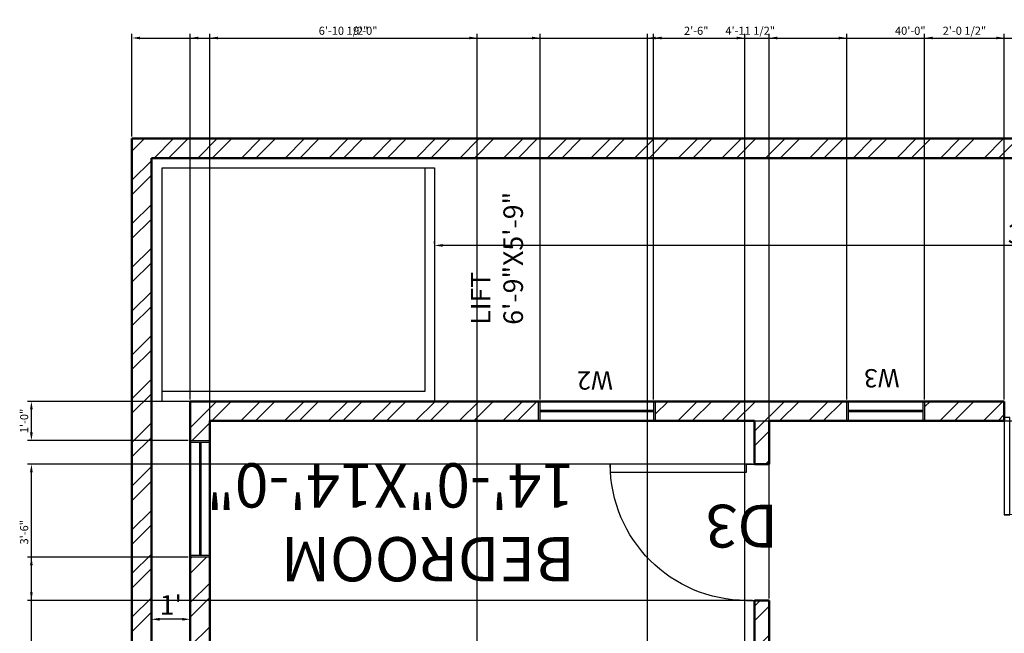
# Model space of a CAD drawing. Units: inches. Extents: x 244 to 2800, y 1060 to 1700.
# Tile 9 of 13: x 1478 to 1781, y 1480 to 1670. Entities that reach past the tile are written whole.
import ezdxf

# ---------------------------------------------------------------- set-up
doc = ezdxf.new("R2010")
doc.units = ezdxf.units.IN
for name, color, linetype, lineweight in [('A-ANNO-DIMS', 2, 'Continuous', 18), ('A-ANNO-TEXT', 1, 'Continuous', 18), ('A-DOOR', 5, 'Continuous', 25), ('A-EQPM', 4, 'Continuous', 25), ('A-GLAZ', 3, 'Continuous', 25), ('A-WALL', 7, 'Continuous', 50), ('A-WALL-PATT', 8, 'Continuous', 13)]:
    doc.layers.add(name, color=color, linetype=linetype, lineweight=lineweight)
doc.styles.get("Standard").update_dxf_attribs({"font": 'arial.ttf'})
doc.dimstyles.new('ISO-25', dxfattribs={"dimtxt": 2.5, "dimasz": 2.5, "dimexe": 1.25, "dimexo": 0.625, "dimtad": 1, "dimlunit": 4, "dimtxsty": 'Standard', "dimcen": 2.5, "dimadec": 0, "dimazin": 0, "dimtfac": 1, "dimtmove": 0, "dimatfit": 3, "dimfxl": 1, "dimarcsym": 0})

# ---------------------------------------------------------------- blocks, each defined once
blk = doc.blocks.new('*U2')
for p, q in [((0, 0), (0, -5)), ((30, 0), (30, -5))]:
    blk.add_line(p, q)
blk.add_lwpolyline([(0, 0), (0, 30), (1.75, 30), (1.75, 0)], close=True)
blk.add_arc((0, 0), 30, 0, 90)
blk = doc.blocks.new('*D29')
at = {"layer": 'A-ANNO-DIMS', "color": 0, "lineweight": -2, "transparency": 16777216}
for p, q in [((1605.7, 1600.68), (1605.7, 1601.31)), ((1983.9, 1600.06), (1608.2, 1600.06)), ((1986.4, 1600.68), (1986.4, 1601.31))]:
    blk.add_line(p, q, dxfattribs=at)
at = {"layer": 'A-ANNO-DIMS', "color": 0, "transparency": 16777216}
for points in [[(1608.2, 1600.47), (1608.2, 1599.64), (1605.7, 1600.06)], [(1983.9, 1600.47), (1983.9, 1599.64), (1986.4, 1600.06)]]:
    blk.add_solid(points, dxfattribs=at)
at = {"layer": 'Defpoints', "color": 0, "transparency": 16777216}
for p in [(1605.7, 1600.06), (1605.7, 1600.06), (1986.4, 1600.06)]:
    blk.add_point(p, dxfattribs=at)
at = {"layer": 'A-ANNO-DIMS', "color": 0, "transparency": 16777216, "insert": (1796.05, 1607.8), "char_height": 6, "attachment_point": 5}
blk.add_mtext('31\'-8{\\H1x;\\S3/4;}"', dxfattribs=at)
blk = doc.blocks.new('*D30')
at = {"layer": 'A-ANNO-DIMS', "color": 0, "lineweight": -2, "transparency": 16777216}
for p, q in [((1518.4, 1482.07), (1518.4, 1486.07)), ((1527.9, 1484.82), (1520.9, 1484.82)), ((1530.4, 1482.07), (1530.4, 1486.07))]:
    blk.add_line(p, q, dxfattribs=at)
at = {"layer": 'A-ANNO-DIMS', "color": 0, "transparency": 16777216}
for points in [[(1520.9, 1485.24), (1520.9, 1484.4), (1518.4, 1484.82)], [(1527.9, 1485.24), (1527.9, 1484.4), (1530.4, 1484.82)]]:
    blk.add_solid(points, dxfattribs=at)
at = {"layer": 'Defpoints', "color": 0, "transparency": 16777216}
for p in [(1518.4, 1484.82), (1518.4, 1481.44), (1530.4, 1481.44)]:
    blk.add_point(p, dxfattribs=at)
at = {"layer": 'A-ANNO-DIMS', "color": 0, "transparency": 16777216, "insert": (1524.4, 1488.46), "char_height": 6, "attachment_point": 5}
blk.add_mtext("1'", dxfattribs=at)
blk = doc.blocks.new('WIN-36')
for p, q in [((0, 0), (0, 6)), ((0, 6), (35.94, 6)), ((35.94, 6), (35.94, 0)), ((35.94, 0), (0, 0))]:
    blk.add_line(p, q)
blk = doc.blocks.new('WIN-24')
for p, q in [((0, 0), (0, 23.94)), ((0, 23.94), (6, 23.94)), ((6, 23.94), (6, 0)), ((6, 0), (0, 0))]:
    blk.add_line(p, q)
blk = doc.blocks.new('LIFT-CAR')
for p, q in [((0, 0), (0, 72)), ((0, 72), (84, 72)), ((81, 72), (81, 3)), ((84, 72), (84, 0)), ((81, 3), (0, 3)), ((84, 0), (0, 0))]:
    blk.add_line(p, q)
blk = doc.blocks.new('*D74')
at = {"layer": 'A-ANNO-DIMS', "color": 0, "lineweight": -2, "transparency": 16777216}
for p, q in [((1512.4, 1633.61), (1512.4, 1665.24)), ((1514.9, 1663.99), (1989.9, 1663.99)), ((1992.4, 1633.61), (1992.4, 1665.24))]:
    blk.add_line(p, q, dxfattribs=at)
at = {"layer": 'A-ANNO-DIMS', "color": 0, "transparency": 16777216}
for points in [[(1514.9, 1664.4), (1514.9, 1663.57), (1512.4, 1663.99)], [(1989.9, 1664.4), (1989.9, 1663.57), (1992.4, 1663.99)]]:
    blk.add_solid(points, dxfattribs=at)
at = {"layer": 'Defpoints', "color": 0, "transparency": 16777216}
for p in [(1992.4, 1663.99), (1512.4, 1632.99), (1992.4, 1632.99)]:
    blk.add_point(p, dxfattribs=at)
at = {"layer": 'A-ANNO-DIMS', "color": 0, "transparency": 16777216, "insert": (1752.4, 1665.89), "char_height": 2.5, "attachment_point": 5}
blk.add_mtext('40\'-0"', dxfattribs=at)
blk = doc.blocks.new('*D76')
at = {"layer": 'A-ANNO-DIMS', "color": 0, "lineweight": -2, "transparency": 16777216}
for p, q in [((1530.4, 1552.61), (1530.4, 1665.24)), ((1532.9, 1663.99), (1635.8, 1663.99)), ((1638.3, 1552.61), (1638.3, 1665.24))]:
    blk.add_line(p, q, dxfattribs=at)
at = {"layer": 'A-ANNO-DIMS', "color": 0, "transparency": 16777216}
for points in [[(1532.9, 1664.4), (1532.9, 1663.57), (1530.4, 1663.99)], [(1635.8, 1664.4), (1635.8, 1663.57), (1638.3, 1663.99)]]:
    blk.add_solid(points, dxfattribs=at)
at = {"layer": 'Defpoints', "color": 0, "transparency": 16777216}
for p in [(1638.3, 1663.99), (1530.4, 1551.99), (1638.3, 1551.99)]:
    blk.add_point(p, dxfattribs=at)
at = {"layer": 'A-ANNO-DIMS', "color": 0, "transparency": 16777216, "insert": (1584.35, 1665.89), "char_height": 2.5, "attachment_point": 5}
blk.add_mtext('9\'-0"', dxfattribs=at)
blk = doc.blocks.new('*D77')
at = {"layer": 'A-ANNO-DIMS', "color": 0, "lineweight": -2, "transparency": 16777216}
for p, q in [((1673.24, 1552.61), (1673.24, 1665.24)), ((1675.74, 1663.99), (1730.36, 1663.99)), ((1732.86, 1552.61), (1732.86, 1665.24))]:
    blk.add_line(p, q, dxfattribs=at)
at = {"layer": 'A-ANNO-DIMS', "color": 0, "transparency": 16777216}
for points in [[(1675.74, 1664.4), (1675.74, 1663.57), (1673.24, 1663.99)], [(1730.36, 1664.4), (1730.36, 1663.57), (1732.86, 1663.99)]]:
    blk.add_solid(points, dxfattribs=at)
at = {"layer": 'Defpoints', "color": 0, "transparency": 16777216}
for p in [(1732.86, 1663.99), (1673.24, 1551.99), (1732.86, 1551.99)]:
    blk.add_point(p, dxfattribs=at)
at = {"layer": 'A-ANNO-DIMS', "color": 0, "transparency": 16777216, "insert": (1703.05, 1665.9), "char_height": 2.5, "attachment_point": 5}
blk.add_mtext('4\'-11 1/2"', dxfattribs=at)
blk = doc.blocks.new('*D78')
at = {"layer": 'A-ANNO-DIMS', "color": 0, "lineweight": -2, "transparency": 16777216}
for p, q in [((1756.81, 1552.61), (1756.81, 1665.24)), ((1759.31, 1663.99), (1778.9, 1663.99)), ((1781.4, 1552.61), (1781.4, 1665.24))]:
    blk.add_line(p, q, dxfattribs=at)
at = {"layer": 'A-ANNO-DIMS', "color": 0, "transparency": 16777216}
for points in [[(1759.31, 1664.4), (1759.31, 1663.57), (1756.81, 1663.99)], [(1778.9, 1664.4), (1778.9, 1663.57), (1781.4, 1663.99)]]:
    blk.add_solid(points, dxfattribs=at)
at = {"layer": 'Defpoints', "color": 0, "transparency": 16777216}
for p in [(1781.4, 1663.99), (1756.81, 1551.99), (1781.4, 1551.99)]:
    blk.add_point(p, dxfattribs=at)
at = {"layer": 'A-ANNO-DIMS', "color": 0, "transparency": 16777216, "insert": (1769.1, 1665.9), "char_height": 2.5, "attachment_point": 5}
blk.add_mtext('2\'-0 1/2"', dxfattribs=at)
blk = doc.blocks.new('*D83')
at = {"layer": 'A-ANNO-DIMS', "color": 0, "lineweight": -2, "transparency": 16777216}
for p, q in [((1529.77, 1503.97), (1480.15, 1503.97)), ((1481.4, 1349.38), (1481.4, 1501.47)), ((1529.77, 1346.88), (1480.15, 1346.88))]:
    blk.add_line(p, q, dxfattribs=at)
at = {"layer": 'A-ANNO-DIMS', "color": 0, "transparency": 16777216}
for points in [[(1480.98, 1501.47), (1481.81, 1501.47), (1481.4, 1503.97)], [(1480.98, 1349.38), (1481.81, 1349.38), (1481.4, 1346.88)]]:
    blk.add_solid(points, dxfattribs=at)
at = {"layer": 'Defpoints', "color": 0, "transparency": 16777216}
for p in [(1481.4, 1503.97), (1530.4, 1503.97), (1530.4, 1346.88)]:
    blk.add_point(p, dxfattribs=at)
at = {"layer": 'A-ANNO-DIMS', "color": 0, "transparency": 16777216, "insert": (1479.49, 1425.42), "char_height": 2.5, "attachment_point": 5, "rotation": 90}
blk.add_mtext('13\'-1"', dxfattribs=at)
blk = doc.blocks.new('*D84')
at = {"layer": 'A-ANNO-DIMS', "color": 0, "lineweight": -2, "transparency": 16777216}
for p, q in [((1529.77, 1551.99), (1480.15, 1551.99)), ((1481.4, 1542.41), (1481.4, 1549.49)), ((1529.77, 1539.91), (1480.15, 1539.91))]:
    blk.add_line(p, q, dxfattribs=at)
at = {"layer": 'A-ANNO-DIMS', "color": 0, "transparency": 16777216}
for points in [[(1480.98, 1549.49), (1481.81, 1549.49), (1481.4, 1551.99)], [(1480.98, 1542.41), (1481.81, 1542.41), (1481.4, 1539.91)]]:
    blk.add_solid(points, dxfattribs=at)
at = {"layer": 'Defpoints', "color": 0, "transparency": 16777216}
for p in [(1481.4, 1551.99), (1530.4, 1551.99), (1530.4, 1539.91)]:
    blk.add_point(p, dxfattribs=at)
at = {"layer": 'A-ANNO-DIMS', "color": 0, "transparency": 16777216, "insert": (1479.49, 1545.95), "char_height": 2.5, "attachment_point": 5, "rotation": 90}
blk.add_mtext('1\'-0"', dxfattribs=at)
blk = doc.blocks.new('*D87')
at = {"layer": 'A-ANNO-DIMS', "color": 0, "lineweight": -2, "transparency": 16777216}
for p, q in [((1537.02, 1545.99), (2024.65, 1545.99)), ((2023.4, 1375.49), (2023.4, 1543.49)), ((1537.02, 1372.99), (2024.65, 1372.99))]:
    blk.add_line(p, q, dxfattribs=at)
at = {"layer": 'A-ANNO-DIMS', "color": 0, "transparency": 16777216}
for points in [[(2022.98, 1543.49), (2023.81, 1543.49), (2023.4, 1545.99)], [(2022.98, 1375.49), (2023.81, 1375.49), (2023.4, 1372.99)]]:
    blk.add_solid(points, dxfattribs=at)
at = {"layer": 'Defpoints', "color": 0, "transparency": 16777216}
for p in [(1536.4, 1545.99), (2023.4, 1545.99), (1536.4, 1372.99)]:
    blk.add_point(p, dxfattribs=at)
at = {"layer": 'A-ANNO-DIMS', "color": 0, "transparency": 16777216, "insert": (2021.49, 1459.49), "char_height": 2.5, "attachment_point": 5, "rotation": 90}
blk.add_mtext('14\'-5"', dxfattribs=at)
blk = doc.blocks.new('*D88')
at = {"layer": 'A-ANNO-DIMS', "color": 0, "lineweight": -2, "transparency": 16777216}
for p, q in [((1536.4, 1373.61), (1536.4, 1665.24)), ((1538.9, 1663.99), (1616.4, 1663.99)), ((1618.9, 1369.11), (1618.9, 1665.24))]:
    blk.add_line(p, q, dxfattribs=at)
at = {"layer": 'A-ANNO-DIMS', "color": 0, "transparency": 16777216}
for points in [[(1538.9, 1664.4), (1538.9, 1663.57), (1536.4, 1663.99)], [(1616.4, 1664.4), (1616.4, 1663.57), (1618.9, 1663.99)]]:
    blk.add_solid(points, dxfattribs=at)
at = {"layer": 'Defpoints', "color": 0, "transparency": 16777216}
for p in [(1618.9, 1663.99), (1536.4, 1372.99), (1618.9, 1368.49)]:
    blk.add_point(p, dxfattribs=at)
at = {"layer": 'A-ANNO-DIMS', "color": 0, "transparency": 16777216, "insert": (1577.65, 1665.9), "char_height": 2.5, "attachment_point": 5}
blk.add_mtext('6\'-10 1/2"', dxfattribs=at)
blk = doc.blocks.new('*D89')
at = {"layer": 'A-ANNO-DIMS', "color": 0, "lineweight": -2, "transparency": 16777216}
for p, q in [((1671.4, 1373.61), (1671.4, 1665.24)), ((1673.9, 1663.99), (1698.9, 1663.99)), ((1701.4, 1373.61), (1701.4, 1665.24))]:
    blk.add_line(p, q, dxfattribs=at)
at = {"layer": 'A-ANNO-DIMS', "color": 0, "transparency": 16777216}
for points in [[(1673.9, 1664.4), (1673.9, 1663.57), (1671.4, 1663.99)], [(1698.9, 1664.4), (1698.9, 1663.57), (1701.4, 1663.99)]]:
    blk.add_solid(points, dxfattribs=at)
at = {"layer": 'Defpoints', "color": 0, "transparency": 16777216}
for p in [(1701.4, 1663.99), (1671.4, 1372.99), (1701.4, 1372.99)]:
    blk.add_point(p, dxfattribs=at)
at = {"layer": 'A-ANNO-DIMS', "color": 0, "transparency": 16777216, "insert": (1686.4, 1665.89), "char_height": 2.5, "attachment_point": 5}
blk.add_mtext('2\'-6"', dxfattribs=at)
blk = doc.blocks.new('*D90')
at = {"layer": 'A-ANNO-DIMS', "color": 0, "lineweight": -2, "transparency": 16777216}
for p, q in [((1708.9, 1491.26), (1708.9, 1665.24)), ((1711.4, 1663.99), (1893.9, 1663.99)), ((1896.4, 1473.26), (1896.4, 1665.24))]:
    blk.add_line(p, q, dxfattribs=at)
at = {"layer": 'A-ANNO-DIMS', "color": 0, "transparency": 16777216}
for points in [[(1711.4, 1664.4), (1711.4, 1663.57), (1708.9, 1663.99)], [(1893.9, 1664.4), (1893.9, 1663.57), (1896.4, 1663.99)]]:
    blk.add_solid(points, dxfattribs=at)
at = {"layer": 'Defpoints', "color": 0, "transparency": 16777216}
for p in [(1896.4, 1663.99), (1708.9, 1490.64), (1896.4, 1472.64)]:
    blk.add_point(p, dxfattribs=at)
at = {"layer": 'A-ANNO-DIMS', "color": 0, "transparency": 16777216, "insert": (1802.65, 1665.9), "char_height": 2.5, "attachment_point": 5}
blk.add_mtext('15\'-7 1/2"', dxfattribs=at)
blk = doc.blocks.new('*D93')
at = {"layer": 'A-ANNO-DIMS', "color": 0, "lineweight": -2, "transparency": 16777216}
for p, q in [((1703.77, 1532.64), (1480.15, 1532.64)), ((1481.4, 1493.14), (1481.4, 1530.14)), ((1703.77, 1490.64), (1480.15, 1490.64))]:
    blk.add_line(p, q, dxfattribs=at)
at = {"layer": 'A-ANNO-DIMS', "color": 0, "transparency": 16777216}
for points in [[(1480.98, 1530.14), (1481.81, 1530.14), (1481.4, 1532.64)], [(1480.98, 1493.14), (1481.81, 1493.14), (1481.4, 1490.64)]]:
    blk.add_solid(points, dxfattribs=at)
at = {"layer": 'Defpoints', "color": 0, "transparency": 16777216}
for p in [(1481.4, 1532.64), (1704.4, 1532.64), (1704.4, 1490.64)]:
    blk.add_point(p, dxfattribs=at)
at = {"layer": 'A-ANNO-DIMS', "color": 0, "transparency": 16777216, "insert": (1479.49, 1511.64), "char_height": 2.5, "attachment_point": 5, "rotation": 90}
blk.add_mtext('3\'-6"', dxfattribs=at)

msp = doc.modelspace()

# ---------------------------------------------------------------- hatches: boundary and pattern name
at = {"layer": 'A-WALL-PATT'}
h = msp.add_hatch(dxfattribs=at)
h.set_pattern_fill('ANSI32', color=256)
h.paths.add_polyline_path([(1992.396, 1092.986), (1992.396, 1632.986), (1512.396, 1632.986), (1512.396, 1092.986)])
h.paths.add_polyline_path([(1518.396, 1098.986), (1518.396, 1626.986), (1986.396, 1626.986), (1986.396, 1098.986), (1902.396, 1098.986)], flags=16)
h.paths.add_polyline_path([(1795.896, 1110.986), (1530.396, 1110.986), (1530.396, 1551.986), (1521.7, 1551.986), (1521.7, 1623.986), (1605.7, 1623.986), (1605.7, 1551.986), (1781.396, 1551.986), (1781.396, 1545.986), (1708.896, 1545.986), (1708.896, 1532.64), (1704.396, 1532.64), (1704.396, 1545.986), (1536.396, 1545.986), (1536.396, 1372.986), (1671.396, 1372.986), (1671.396, 1368.486), (1621.896, 1368.486), (1621.896, 1296.486), (1704.396, 1296.486), (1704.396, 1368.486), (1701.396, 1368.486), (1701.396, 1372.986), (1704.396, 1372.986), (1704.396, 1490.64), (1708.896, 1490.64), (1708.896, 1288.986), (1704.396, 1288.986), (1704.396, 1291.986), (1569.396, 1291.986), (1569.396, 1296.486), (1618.896, 1296.486), (1618.896, 1368.486), (1536.396, 1368.486), (1536.396, 1296.486), (1539.396, 1296.486), (1539.396, 1291.986), (1536.396, 1291.986), (1536.396, 1116.986), (1704.396, 1116.986), (1704.396, 1246.986), (1708.896, 1246.986), (1708.896, 1116.986), (1744.896, 1116.986), (1744.896, 1260.986), (1780.896, 1260.986), (1785.396, 1260.986), (1785.396, 1205.486), (1831.896, 1205.486), (1831.896, 1217.486), (1836.396, 1217.486), (1836.396, 1205.486), (1896.396, 1205.486), (1896.396, 1265.486), (1836.396, 1265.486), (1836.396, 1253.486), (1831.896, 1253.486), (1831.896, 1269.986), (1896.396, 1269.986), (1896.396, 1472.64), (1902.396, 1472.64), (1902.396, 1242.986), (1938.396, 1242.986), (1938.396, 1134.986), (1950.396, 1134.986), (1950.396, 1242.986), (1986.396, 1242.986), (1986.396, 1134.986), (1902.396, 1134.986), (1902.396, 1110.986), (1831.896, 1110.986), (1831.896, 1116.986), (1896.396, 1116.986), (1896.396, 1200.986), (1785.396, 1200.986), (1785.396, 1116.986), (1795.896, 1116.986)], flags=0)
h.paths.add_polyline_path([(1780.896, 1116.986), (1744.896, 1116.986), (1744.896, 1260.986), (1780.896, 1260.986)], flags=0)
h.paths.add_polyline_path([(1863.351, 1110.986), (1863.351, 1116.986), (1887.296, 1116.986), (1887.296, 1110.986)], flags=0)
h.paths.add_polyline_path([(1863.851, 1114.186), (1886.796, 1114.186), (1886.796, 1113.786), (1863.851, 1113.786)], flags=0)
h.paths.add_polyline_path([(1896.396, 1174.102), (1896.396, 1198.047), (1902.396, 1198.047), (1902.396, 1174.102)], flags=0)
h.paths.add_polyline_path([(1902.396, 1174.602), (1899.196, 1174.602), (1899.196, 1197.547), (1902.396, 1197.547)], flags=0)
h.paths.add_polyline_path([(1692.519, 1110.986), (1656.574, 1110.986), (1656.574, 1116.986), (1692.519, 1116.986)], flags=0)
h.paths.add_polyline_path([(1819.776, 1376.187), (1819.776, 1410.382, -0.249194), (1838.546, 1410.382), (1838.546, 1376.187, -0.249194)], flags=0)
h.paths.add_polyline_path([(1536.396, 1250.972), (1530.396, 1250.972), (1530.396, 1286.917), (1536.396, 1286.917)], flags=0)
h.paths.add_polyline_path([(1896.396, 1405.581), (1896.396, 1453.526), (1902.396, 1453.526), (1902.396, 1405.581)], flags=0)
h.paths.add_polyline_path([(1536.396, 1322.935), (1530.396, 1322.935), (1530.396, 1346.88), (1536.396, 1346.88)], flags=0)
h.paths.add_polyline_path([(1533.196, 1323.435), (1533.196, 1346.38), (1533.596, 1346.38), (1533.596, 1323.435)], flags=0)
h.paths.add_polyline_path([(1896.396, 1545.986), (1841.396, 1545.986), (1841.396, 1551.986), (1902.396, 1551.986), (1902.396, 1532.64), (1896.396, 1532.64)], flags=0)
h.paths.add_polyline_path([(1756.808, 1545.986), (1732.863, 1545.986), (1732.863, 1551.986), (1756.808, 1551.986)], flags=0)
h.paths.add_polyline_path([(1756.308, 1548.786), (1733.363, 1548.786), (1733.363, 1551.986), (1756.308, 1551.986)], flags=0)
h.paths.add_polyline_path([(1673.743, 1545.986), (1637.798, 1545.986), (1637.798, 1551.986), (1673.743, 1551.986)], flags=0)
h.paths.add_polyline_path([(1536.396, 1503.969), (1530.396, 1503.969), (1530.396, 1539.914), (1536.396, 1539.914)], flags=0)
h.paths.add_polyline_path([(1896.341, 1192.868), (1881.737, 1192.868), (1881.737, 1181.273), (1896.341, 1181.273)], flags=8)
h.paths.add_polyline_path([(1882.893, 1112.542), (1868.29, 1112.542), (1868.29, 1100.947), (1882.893, 1100.947)], flags=8)
h.paths.add_polyline_path([(1531.898, 1340.208), (1517.295, 1340.208), (1517.295, 1328.613), (1531.898, 1328.613)], flags=24)
h.paths.add_polyline_path([(1662.207, 1564.332), (1647.603, 1564.332), (1647.603, 1552.737), (1662.207, 1552.737)], flags=8)
h.paths.add_polyline_path([(1750.605, 1565.018), (1736.001, 1565.018), (1736.001, 1553.424), (1750.605, 1553.424)], flags=8)
h.paths.add_polyline_path([(1919.351, 1440.326), (1904.748, 1440.326), (1904.748, 1428.731), (1919.351, 1428.731)], flags=8)
h.paths.add_polyline_path([(1827.662, 1149.994), (1797.512, 1149.994), (1797.512, 1122.813), (1827.662, 1122.813)], flags=8)
h.paths.add_polyline_path([(1826.683, 1247.85), (1796.533, 1247.85), (1796.533, 1220.668), (1826.683, 1220.668)], flags=8)
h.paths.add_polyline_path([(1713.043, 1285.137), (1682.893, 1285.137), (1682.893, 1257.956), (1713.043, 1257.956)], flags=8)
h.paths.add_polyline_path([(1567.301, 1310.129), (1537.151, 1310.129), (1537.151, 1282.948), (1567.301, 1282.948)], flags=8)
h.paths.add_polyline_path([(1699.655, 1386.046), (1669.505, 1386.046), (1669.505, 1358.865), (1699.655, 1358.865)], flags=8)
h.paths.add_polyline_path([(1716.254, 1527.375), (1686.103, 1527.375), (1686.103, 1500.194), (1716.254, 1500.194)], flags=8)
h.paths.add_polyline_path([(1822.088, 1577.207), (1791.938, 1577.207), (1791.938, 1550.026), (1822.088, 1550.026)], flags=8)
h.paths.add_polyline_path([(1931.716, 1518.23), (1901.565, 1518.23), (1901.565, 1491.049), (1931.716, 1491.049)], flags=8)
h.paths.add_polyline_path([(1636.272, 1573.477), (1636.272, 1615.869), (1613.819, 1615.869), (1613.819, 1573.477)], flags=8)
h.paths.add_polyline_path([(1968.141, 1266.003), (1911.144, 1266.003), (1911.144, 1252.05), (1968.141, 1252.05)], flags=8)
h.paths.add_polyline_path([(1783.26, 1275.202), (1745.711, 1275.202), (1745.711, 1261.249), (1783.26, 1261.249)], flags=8)
h.paths.add_polyline_path([(1753.522, 1456.095), (1753.522, 1338.024), (1798.876, 1338.024), (1798.876, 1456.095)], flags=8)
h.paths.add_polyline_path([(1884.04, 1192.467), (1803.345, 1192.467), (1803.345, 1149.693), (1884.04, 1149.693)], flags=8)
h.paths.add_polyline_path([(1863.426, 1264.753), (1863.426, 1209.557), (1892.661, 1209.557), (1892.661, 1264.753)], flags=8)
h.paths.add_polyline_path([(1594.411, 1361.178), (1536.688, 1361.178), (1536.688, 1330.387), (1594.411, 1330.387)], flags=8)
h.paths.add_polyline_path([(1695.984, 1342.402), (1638.262, 1342.402), (1638.262, 1311.611), (1695.984, 1311.611)], flags=8)
h.paths.add_polyline_path([(1654.435, 1540.65), (1537.752, 1540.65), (1537.752, 1489.721), (1654.435, 1489.721)], flags=8)
h.paths.add_polyline_path([(1658.864, 1271.272), (1542.182, 1271.272), (1542.182, 1220.343), (1658.864, 1220.343)], flags=8)
h = msp.add_hatch(dxfattribs=at)
h.set_pattern_fill('ANSI32', color=256)
h.paths.add_polyline_path([(1637.798, 1551.986), (1530.396, 1551.986), (1530.396, 1539.914), (1536.396, 1539.914), (1536.396, 1545.986), (1637.798, 1545.986)])
h = msp.add_hatch(dxfattribs=at)
h.set_pattern_fill('ANSI32', color=256)
h.paths.add_polyline_path([(1732.863, 1551.986), (1673.743, 1551.986), (1673.743, 1545.986), (1704.396, 1545.986), (1704.396, 1532.64), (1708.896, 1532.64), (1708.896, 1545.986), (1711.896, 1545.986), (1732.863, 1545.986)])
h = msp.add_hatch(dxfattribs=at)
h.set_pattern_fill('ANSI32', color=256)
h.paths.add_polyline_path([(1781.396, 1551.986), (1756.808, 1551.986), (1756.808, 1545.986), (1781.396, 1545.986), (1781.396, 1546.986)])
h = msp.add_hatch(dxfattribs=at)
h.set_pattern_fill('ANSI32', color=256)
h.paths.add_polyline_path([(1708.896, 1490.64), (1704.396, 1490.64), (1704.396, 1372.986), (1701.396, 1372.986), (1701.396, 1368.486), (1704.396, 1368.486), (1704.396, 1296.486), (1621.896, 1296.486), (1621.896, 1368.486), (1671.396, 1368.486), (1671.396, 1372.986), (1536.396, 1372.986), (1536.396, 1503.969), (1530.396, 1503.969), (1530.396, 1346.88), (1536.396, 1346.88), (1536.396, 1368.486), (1618.896, 1368.486), (1618.896, 1296.486), (1569.396, 1296.486), (1569.396, 1291.986), (1572.396, 1291.986), (1704.396, 1291.986), (1704.396, 1288.986), (1708.896, 1288.986)])

# ---------------------------------------------------------------- linework, layer by layer
at = {"layer": 'A-GLAZ'}
for p, q in [((1638.298, 1545.986), (1638.298, 1551.986)), ((1673.243, 1551.986), (1673.243, 1545.986)), ((1733.363, 1545.986), (1733.363, 1551.986)), ((1756.308, 1551.986), (1756.308, 1545.986)), ((1673.243, 1549.186), (1638.298, 1549.186)), ((1673.243, 1548.786), (1638.298, 1548.786)), ((1756.308, 1549.186), (1733.363, 1549.186)), ((1756.308, 1548.786), (1733.363, 1548.786)), ((1530.396, 1539.414), (1536.396, 1539.414)), ((1533.196, 1539.414), (1533.196, 1504.469)), ((1533.596, 1539.414), (1533.596, 1504.469)), ((1536.396, 1504.469), (1530.396, 1504.469))]:
    msp.add_line(p, q, dxfattribs=at)
at = {"layer": 'A-WALL'}
for p, q in [((1992.396, 1632.986), (1512.396, 1632.986)), ((1512.396, 1632.986), (1512.396, 1092.986)), ((1518.396, 1626.986), (1518.396, 1098.986)), ((1986.396, 1626.986), (1518.396, 1626.986)), ((1530.396, 1551.986), (1530.396, 1110.986)), ((1530.396, 1551.986), (1781.396, 1551.986)), ((1711.896, 1551.986), (1771.896, 1551.986)), ((1781.396, 1551.986), (1781.396, 1545.986)), ((1536.396, 1545.986), (1536.396, 1372.986)), ((1536.396, 1545.986), (1704.396, 1545.986)), ((1704.396, 1545.986), (1704.396, 1532.64)), ((1708.896, 1545.986), (1708.896, 1532.64)), ((1708.896, 1545.986), (1711.896, 1545.986)), ((1708.896, 1545.986), (1781.396, 1545.986)), ((1708.896, 1532.64), (1704.396, 1532.64)), ((1704.396, 1490.64), (1708.896, 1490.64)), ((1704.396, 1490.64), (1704.396, 1372.986)), ((1708.896, 1490.64), (1708.896, 1288.986))]:
    msp.add_line(p, q, dxfattribs=at)

# ---------------------------------------------------------------- block references
at = {"layer": 'A-DOOR'}
for p, xscale, yscale, zscale, rotation in [((1781.396, 1546.986), -0.9999956819955501, 0.9999956819955501, 0.9999956819955501, 180), ((1701.896, 1532.64), -1.399999999999999, 1.399999999999999, 1.399999999999999, 90)]:
    msp.add_blockref('*U2', p, dxfattribs=dict(at, xscale=xscale, yscale=yscale, zscale=zscale, rotation=rotation))
at = {"layer": 'A-EQPM'}
msp.add_blockref('LIFT-CAR', (1521.7, 1551.986), dxfattribs=at)
at = {"layer": 'A-GLAZ'}
msp.add_blockref('WIN-36', (1637.798, 1545.986), dxfattribs=at)
for name, p, rotation in [('WIN-24', (1756.808, 1545.986), 90.00000000000126), ('WIN-36', (1530.396, 1539.914), 269.9999999999988)]:
    msp.add_blockref(name, p, dxfattribs=dict(at, rotation=rotation))

# ---------------------------------------------------------------- texts
at = {"layer": 'A-ANNO-TEXT', "attachment_point": 1}
for s, width, gutter_width, insert, char_height, rotation in [('LIFT\\P6\'-9"X5\'-9"', 12.02436, 30.086, (1616.916, 1575.597), 6.01727, 90), ('W2', 2.91536, 28.132, (1660.704, 1555.61), 5.6265, 180), ('W3', 2.91536, 28.132, (1749.102, 1556.296), 5.6265, 180), ('BEDROOM\\P14\'-0"X14\'-0"', 25.27039, 68.243, (1648.946, 1496.503), 13.64851, 180), ('D3', 20.58737, 65.951, (1711.535, 1506.929), 13.1902, 180)]:
    msp.add_mtext_dynamic_manual_height_columns(s, width=width, gutter_width=gutter_width, heights=[0], dxfattribs=dict(at, insert=insert, char_height=char_height, rotation=rotation))

# ---------------------------------------------------------------- dimensions: what is measured, and where the dimension line sits
at = {"layer": 'A-ANNO-DIMS'}
for base, p1, p2, override, picture, middle in [((1992.396, 1663.986), (1512.396, 1632.986), (1992.396, 1632.986), {"dimdec": 1, "dimlfac": 1, "dimrnd": 0, "dimzin": 1, "dimdsep": 46, "dimlunit": 4, "dimfrac": 2}, '*D74', (1752.396, 1665.888)), ((1638.298, 1663.986), (1530.396, 1551.986), (1638.298, 1551.986), {"dimdec": 1, "dimlfac": 1, "dimrnd": 0, "dimzin": 1, "dimdsep": 46, "dimlunit": 4, "dimfrac": 2}, '*D76', (1584.347, 1665.888)), ((1618.896, 1663.986), (1536.396, 1372.986), (1618.896, 1368.486), {"dimdec": 1, "dimlfac": 1, "dimrnd": 0, "dimzin": 1, "dimdsep": 46, "dimlunit": 4, "dimfrac": 2}, '*D88', (1577.646, 1665.904)), ((1701.396, 1663.986), (1671.396, 1372.986), (1701.396, 1372.986), {"dimdec": 1, "dimlfac": 1, "dimrnd": 0, "dimzin": 1, "dimdsep": 46, "dimlunit": 4, "dimfrac": 2}, '*D89', (1686.396, 1665.888)), ((1732.863, 1663.986), (1673.243, 1551.986), (1732.863, 1551.986), {"dimdec": 1, "dimlfac": 1, "dimrnd": 0, "dimzin": 1, "dimdsep": 46, "dimlunit": 4, "dimfrac": 2}, '*D77', (1703.053, 1665.904)), ((1896.396, 1663.986), (1708.896, 1490.64), (1896.396, 1472.64), {"dimdec": 1, "dimlfac": 1, "dimrnd": 0, "dimzin": 1, "dimdsep": 46, "dimlunit": 4, "dimfrac": 2}, '*D90', (1802.646, 1665.904)), ((1781.396, 1663.986), (1756.808, 1551.986), (1781.396, 1551.986), {"dimdec": 1, "dimlfac": 1, "dimrnd": 0, "dimzin": 1, "dimdsep": 46, "dimlunit": 4, "dimfrac": 2}, '*D78', (1769.102, 1665.904)), ((1605.7, 1600.057), (1986.396, 1600.057), (1605.7, 1600.057), {"dimtxt": 6, "dimclrd": 0, "dimclre": 0, "dimclrt": 0}, '*D29', (1796.048, 1607.8)), ((1518.396, 1484.82), (1530.396, 1481.444), (1518.396, 1481.444), {"dimtxt": 6, "dimclrd": 0, "dimclre": 0, "dimclrt": 0}, '*D30', (1524.396, 1488.457))]:
    dim = msp.add_linear_dim(base=base, p1=p1, p2=p2, dimstyle='ISO-25', override=override, dxfattribs=at)
    dim.commit()
    dim.dimension.update_dxf_attribs({"geometry": picture, "text_midpoint": middle})
for base, p1, p2, picture, middle in [((1481.396, 1551.986), (1530.396, 1539.914), (1530.396, 1551.986), '*D84', (1479.494, 1545.95)), ((2023.396, 1545.986), (1536.396, 1372.986), (1536.396, 1545.986), '*D87', (2021.494, 1459.486)), ((1481.396, 1532.64), (1704.396, 1490.64), (1704.396, 1532.64), '*D93', (1479.493, 1511.64)), ((1481.396, 1503.969), (1530.396, 1346.88), (1530.396, 1503.969), '*D83', (1479.493, 1425.425))]:
    dim = msp.add_linear_dim(base=base, p1=p1, p2=p2, angle=90, dimstyle='ISO-25', override={"dimdec": 1, "dimlfac": 1, "dimrnd": 0, "dimzin": 1, "dimdsep": 46, "dimlunit": 4, "dimfrac": 2}, dxfattribs=at)
    dim.commit()
    dim.dimension.update_dxf_attribs({"geometry": picture, "text_midpoint": middle})

doc.saveas('drawing.dxf')
